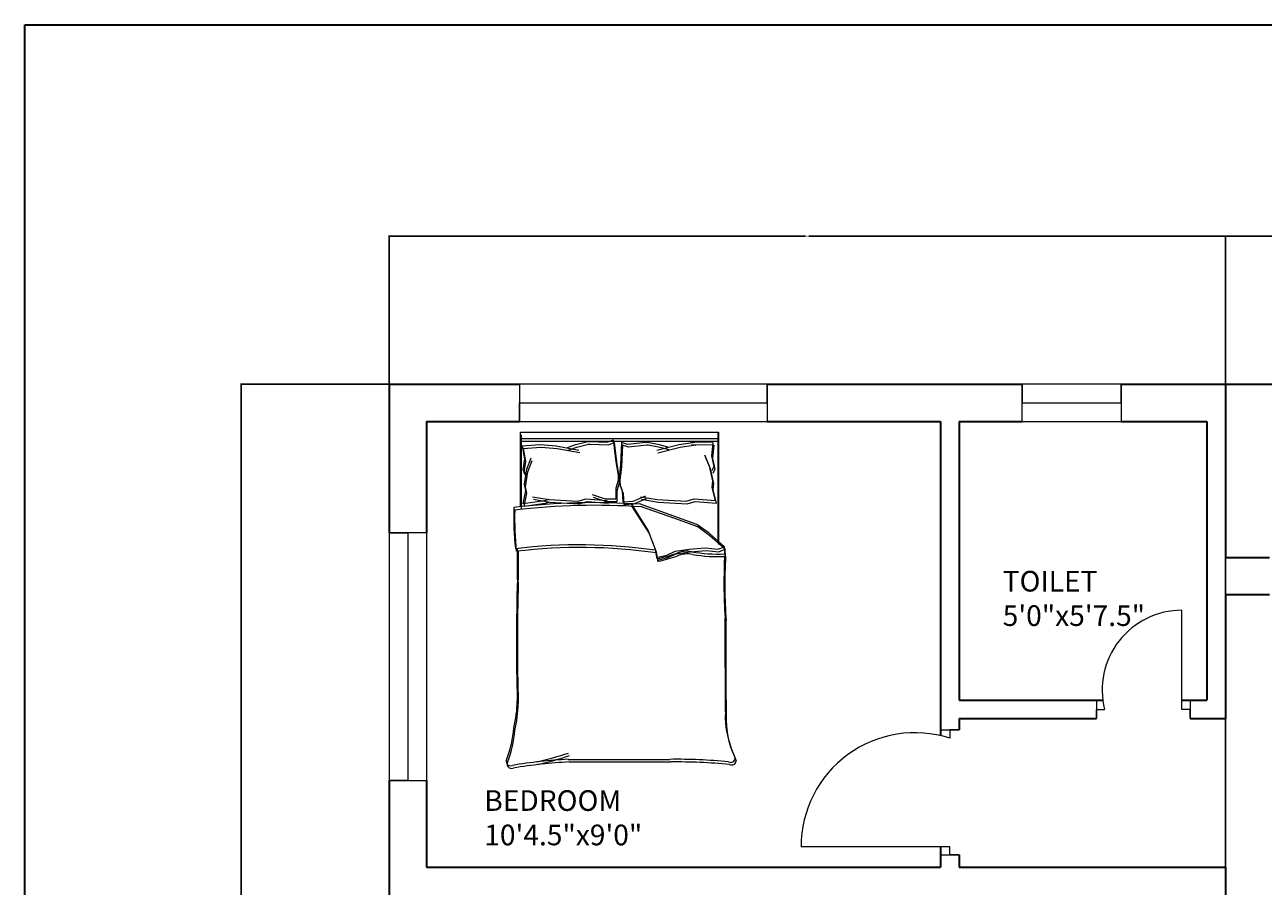
# Model space of a CAD drawing. Units: inches. Extents: x 2527 to 3140, y 1564 to 2435.
# Tile 3 of 4: x 2527 to 2827, y 2227 to 2435. Entities that reach past the tile are written whole.
import ezdxf

# ---------------------------------------------------------------- set-up
doc = ezdxf.new("R2010")
doc.units = ezdxf.units.IN
for name, color, linetype, lineweight in [('A-ANNO-DIMS', 2, 'Continuous', 18), ('A-ANNO-TTLB', 7, 'Continuous', 35), ('A-AREA-IDEN', 7, 'Continuous', 18), ('A-DOOR', 191, 'Continuous', 18), ('A-FURN', 8, 'Continuous', 13), ('A-GLAZ', 131, 'Continuous', 18), ('A-WALL', 7, 'Continuous', 35)]:
    doc.layers.add(name, color=color, linetype=linetype, lineweight=lineweight)
doc.styles.get("Standard").update_dxf_attribs({"font": 'arial.ttf'})
doc.dimstyles.get("Standard").update_dxf_attribs({"dimtxt": 0.18, "dimasz": 0.18, "dimexe": 0.18, "dimexo": 0.0625, "dimgap": 0.09, "dimtad": 0, "dimtih": 1, "dimtoh": 1, "dimdec": 4, "dimzin": 0, "dimdsep": 46, "dimtxsty": 'Standard', "dimcen": 0.09, "dimadec": 0, "dimazin": 0, "dimtfac": 1, "dimtdec": 4, "dimtofl": 0, "dimtmove": 0, "dimatfit": 3, "dimfxl": 1, "dimtolj": 1, "dimtzin": 0, "dimarcsym": 0})

# ---------------------------------------------------------------- blocks, each defined once
blk = doc.blocks.new('BED-DOUBLE')
for p, q in [((3.48, 63.33), (3.48, 81.44)), ((3.48, 63.33), (3.48, 81.44)), ((3.48, 81.44), (51.49, 81.44)), ((51.27, 81.44), (51.27, 54.83)), ((51.27, 81.44), (51.27, 54.83)), ((51.49, 81.44), (51.49, 80.8)), ((3.48, 79.91), (51.27, 79.91)), ((3.48, 79.91), (51.27, 79.91)), ((3.7, 62.69), (3.7, 80.8)), ((3.7, 62.69), (3.7, 80.8)), ((3.7, 79.27), (51.49, 79.27)), ((3.7, 79.27), (51.49, 79.27)), ((3.89, 78.13), (4.47, 74.95)), ((3.9, 78.1), (8.18, 78.43)), ((3.9, 78.1), (8.18, 78.43)), ((3.9, 78.13), (4.47, 74.95)), ((8.18, 78.43), (8.29, 78.42)), ((8.18, 78.43), (8.29, 78.42)), ((8.29, 78.42), (12.11, 78.13)), ((8.29, 78.42), (12.11, 78.13)), ((12.11, 78.13), (17.6, 77.11)), ((12.11, 78.13), (17.6, 77.11)), ((14.86, 77.69), (16.88, 78.42)), ((14.86, 77.69), (16.88, 78.42)), ((16.88, 78.42), (19.77, 79.14)), ((16.88, 78.42), (19.77, 79.14)), ((17.11, 77.78), (20, 78.5)), ((17.11, 77.78), (20, 78.5)), ((19.77, 79.14), (20.09, 79.14)), ((19.77, 79.14), (20.09, 79.14)), ((20, 78.5), (20.32, 78.5)), ((20, 78.5), (20.32, 78.5)), ((20.09, 79.14), (24.54, 78.99)), ((20.09, 79.14), (24.54, 78.99)), ((20.32, 78.5), (24.77, 78.35)), ((20.32, 78.5), (24.77, 78.35)), ((24.54, 78.99), (25.98, 79.57)), ((24.54, 78.99), (25.98, 79.57)), ((24.77, 78.35), (26.21, 78.93)), ((24.77, 78.35), (26.21, 78.93)), ((25.98, 79.57), (26.56, 74.22)), ((25.98, 79.57), (26.56, 74.22)), ((26.21, 78.93), (26.79, 73.58)), ((26.21, 78.93), (26.79, 73.58)), ((27.98, 78.95), (27.73, 73.58)), ((27.98, 78.95), (27.73, 73.58)), ((28.21, 78.31), (27.96, 72.94)), ((28.21, 78.31), (27.96, 72.94)), ((29.46, 78.46), (27.98, 78.95)), ((29.46, 78.46), (27.98, 78.95)), ((29.68, 77.82), (28.21, 78.31)), ((29.68, 77.82), (28.21, 78.31)), ((33.88, 78.89), (29.46, 78.46)), ((33.88, 78.89), (29.46, 78.46)), ((34.11, 78.25), (29.68, 77.82)), ((34.11, 78.25), (29.68, 77.82)), ((34.21, 78.91), (33.88, 78.89)), ((34.2, 78.91), (33.88, 78.89)), ((34.43, 78.27), (34.11, 78.25)), ((34.43, 78.27), (34.11, 78.25)), ((37.14, 78.36), (34.2, 78.91)), ((37.14, 78.36), (34.21, 78.91)), ((37.36, 77.73), (34.43, 78.27)), ((37.36, 77.73), (34.43, 78.27)), ((41.91, 78.37), (36.5, 77.02)), ((41.91, 78.37), (36.5, 77.02)), ((39.2, 77.77), (37.14, 78.36)), ((39.2, 77.77), (37.14, 78.36)), ((45.71, 78.9), (41.91, 78.37)), ((45.71, 78.9), (41.91, 78.37)), ((45.94, 78.26), (42.14, 77.73)), ((45.94, 78.26), (42.14, 77.73)), ((50.11, 78.89), (44.71, 78.98)), ((44.71, 78.98), (45.71, 78.9)), ((50.11, 78.89), (44.71, 78.98)), ((44.71, 78.98), (45.71, 78.9)), ((50.34, 78.25), (44.94, 78.34)), ((44.94, 78.34), (45.94, 78.26)), ((50.34, 78.25), (44.94, 78.34)), ((44.94, 78.34), (45.94, 78.26)), ((50.11, 78.89), (49.73, 75.68)), ((50.11, 78.89), (49.73, 75.68)), ((50.34, 78.25), (49.96, 75.04)), ((50.34, 78.25), (49.96, 75.04)), ((51.49, 80.8), (51.49, 54.19)), ((51.49, 80.8), (51.49, 54.19)), ((4.12, 77.49), (4.7, 74.31)), ((4.12, 77.49), (4.7, 74.31)), ((4.13, 77.47), (8.41, 77.79)), ((4.13, 77.47), (8.41, 77.79)), ((5.05, 72.49), (6.06, 75.24)), ((5.05, 72.49), (6.06, 75.24)), ((8.41, 77.79), (8.51, 77.78)), ((8.41, 77.79), (8.51, 77.78)), ((8.51, 77.78), (12.34, 77.49)), ((8.51, 77.78), (12.34, 77.49)), ((12.34, 77.49), (17.83, 76.48)), ((12.34, 77.49), (17.83, 76.48)), ((15.08, 77.05), (17.11, 77.78)), ((15.08, 77.05), (17.11, 77.78)), ((42.14, 77.73), (36.72, 76.38)), ((42.14, 77.73), (36.72, 76.38)), ((39.43, 77.13), (37.36, 77.73)), ((39.43, 77.13), (37.36, 77.73)), ((49.31, 73.19), (48.13, 75.86)), ((49.31, 73.19), (48.13, 75.86)), ((49.54, 72.55), (48.36, 75.23)), ((49.54, 72.55), (48.36, 75.23)), ((49.73, 75.68), (50.33, 73.1)), ((49.73, 75.68), (50.33, 73.1)), ((49.96, 75.04), (50.56, 72.47)), ((49.96, 75.04), (50.56, 72.47)), ((4.47, 74.95), (4.04, 72.34)), ((4.47, 74.95), (4.04, 72.34)), ((4.04, 72.34), (4.62, 71.33)), ((4.04, 72.34), (4.62, 71.33)), ((4.7, 74.31), (4.27, 71.7)), ((4.7, 74.31), (4.27, 71.7)), ((4.47, 68.87), (5.05, 72.49)), ((4.47, 68.87), (5.05, 72.49)), ((5.28, 71.85), (6.29, 74.6)), ((5.28, 71.85), (6.29, 74.6)), ((26.56, 74.22), (27.14, 71.04)), ((26.56, 74.22), (27.14, 71.04)), ((26.79, 73.58), (27.37, 70.4)), ((26.79, 73.58), (27.37, 70.4)), ((27.73, 73.58), (27.36, 70.36)), ((27.73, 73.58), (27.36, 70.36)), ((27.96, 72.94), (27.58, 69.73)), ((27.96, 72.94), (27.58, 69.73)), ((50.11, 69.61), (49.31, 73.19)), ((50.11, 69.61), (49.31, 73.19)), ((50.34, 68.97), (49.54, 72.55)), ((50.34, 68.97), (49.54, 72.55)), ((50.33, 73.1), (49.81, 72.06)), ((50.33, 73.1), (49.82, 72.06)), ((50.56, 72.47), (50.04, 71.42)), ((50.56, 72.47), (50.04, 71.42)), ((4.27, 71.7), (4.85, 70.69)), ((4.27, 71.7), (4.85, 70.69)), ((4.7, 68.23), (5.28, 71.85)), ((4.7, 68.23), (5.28, 71.85)), ((27.14, 69.74), (26.56, 67.86)), ((27.14, 69.74), (26.56, 67.86)), ((27.37, 69.1), (26.79, 67.22)), ((27.37, 69.1), (26.79, 67.22)), ((27.14, 71.04), (27.14, 69.74)), ((27.14, 71.04), (27.14, 69.74)), ((27.36, 70.36), (27.44, 69.07)), ((27.36, 70.36), (27.44, 69.07)), ((27.37, 70.4), (27.37, 69.1)), ((27.37, 70.4), (27.37, 69.1)), ((27.44, 69.07), (28.13, 67.23)), ((27.44, 69.07), (28.13, 67.23)), ((27.58, 69.73), (27.66, 68.43)), ((27.58, 69.73), (27.66, 68.43)), ((49.92, 68.01), (50.11, 69.61)), ((49.92, 68.01), (50.11, 69.61)), ((4.18, 64.1), (4.76, 67.28)), ((4.18, 64.1), (4.76, 67.28)), ((4.41, 63.46), (4.99, 66.64)), ((4.41, 63.46), (4.99, 66.64)), ((4.76, 67.28), (4.47, 68.87)), ((4.76, 67.28), (4.47, 68.87)), ((4.99, 66.64), (4.7, 68.23)), ((4.99, 66.64), (4.7, 68.23)), ((24.1, 65.18), (20.96, 66.27)), ((24.1, 65.18), (20.96, 66.27)), ((26.56, 67.86), (26.56, 65.18)), ((26.56, 67.86), (26.56, 65.18)), ((26.79, 67.22), (26.79, 64.54)), ((26.79, 67.22), (26.79, 64.54)), ((27.66, 68.43), (28.36, 66.59)), ((27.66, 68.43), (28.36, 66.59)), ((28.13, 67.23), (28.3, 64.55)), ((28.13, 67.23), (28.3, 64.55)), ((28.36, 66.59), (28.53, 63.91)), ((28.36, 66.59), (28.53, 63.91)), ((50.7, 64.87), (49.92, 68.01)), ((50.7, 64.87), (49.92, 68.01)), ((50.15, 67.37), (50.34, 68.97)), ((50.15, 67.37), (50.34, 68.97)), ((50.93, 64.23), (50.15, 67.37)), ((50.93, 64.23), (50.15, 67.37)), ((9.28, 64.82), (4.18, 64.1)), ((9.28, 64.82), (4.18, 64.1)), ((9.51, 64.19), (4.41, 63.46)), ((9.51, 64.19), (4.41, 63.46)), ((6.38, 65.81), (10.41, 65.15)), ((6.38, 65.81), (10.41, 65.15)), ((6.61, 65.17), (10.64, 64.51)), ((6.61, 65.17), (10.64, 64.51)), ((10.41, 65.15), (9.28, 64.82)), ((10.41, 65.15), (9.28, 64.82)), ((10.64, 64.51), (9.51, 64.19)), ((10.64, 64.51), (9.51, 64.19)), ((10.41, 65.15), (17.42, 64.72)), ((10.41, 65.15), (17.42, 64.72)), ((10.64, 64.51), (17.65, 64.08)), ((10.64, 64.51), (17.65, 64.08)), ((17.42, 64.72), (19.38, 65.27)), ((17.42, 64.72), (19.38, 65.27)), ((17.65, 64.08), (19.61, 64.63)), ((17.65, 64.08), (19.61, 64.63)), ((19.38, 65.27), (24.52, 64.87)), ((19.38, 65.27), (24.52, 64.87)), ((19.61, 64.63), (24.74, 64.23)), ((19.61, 64.63), (24.74, 64.23)), ((24.33, 64.54), (21.19, 65.63)), ((24.33, 64.54), (21.19, 65.63)), ((26.56, 65.18), (24.1, 65.18)), ((26.56, 65.18), (24.1, 65.18)), ((26.79, 64.54), (24.33, 64.54)), ((26.79, 64.54), (24.33, 64.54)), ((28.3, 64.55), (30.75, 64.7)), ((28.3, 64.55), (30.75, 64.7)), ((28.53, 63.91), (30.98, 64.06)), ((28.53, 63.91), (30.98, 64.06)), ((30.26, 64.06), (34.45, 57.57)), ((30.26, 64.06), (34.45, 57.57)), ((30.49, 63.42), (34.68, 56.93)), ((30.49, 63.42), (34.68, 56.93)), ((30.75, 64.7), (33.82, 65.99)), ((30.75, 64.7), (33.82, 65.99)), ((30.98, 64.06), (34.05, 65.35)), ((30.98, 64.06), (34.05, 65.35)), ((40.64, 61.13), (32.31, 64.06)), ((40.64, 61.13), (32.31, 64.06)), ((40.87, 60.49), (32.53, 63.42)), ((40.87, 60.49), (32.54, 63.42)), ((32.56, 65.81), (36.6, 65.15)), ((32.56, 65.81), (36.6, 65.15)), ((32.79, 65.17), (36.83, 64.51)), ((32.79, 65.17), (36.82, 64.51)), ((36.6, 65.15), (43.61, 64.72)), ((36.6, 65.15), (43.61, 64.72)), ((36.82, 64.51), (43.83, 64.08)), ((36.83, 64.51), (43.84, 64.08)), ((43.61, 64.72), (45.57, 65.27)), ((43.61, 64.72), (45.57, 65.27)), ((43.83, 64.08), (45.8, 64.63)), ((43.84, 64.08), (45.8, 64.63)), ((45.57, 65.27), (50.7, 64.87)), ((45.57, 65.27), (50.7, 64.87)), ((45.8, 64.63), (50.93, 64.23)), ((45.8, 64.63), (50.93, 64.23)), ((46.22, 59.11), (40.64, 61.13)), ((46.22, 59.11), (40.64, 61.13)), ((46.45, 58.47), (40.87, 60.49)), ((46.45, 58.47), (40.87, 60.49)), ((34.45, 57.57), (36.15, 53.08)), ((34.45, 57.57), (36.15, 53.08)), ((49.16, 56.95), (46.22, 59.11)), ((49.16, 56.95), (46.22, 59.11)), ((49.39, 56.31), (46.45, 58.47)), ((49.39, 56.31), (46.45, 58.47)), ((34.68, 56.93), (36.38, 52.44)), ((34.68, 56.93), (36.38, 52.44)), ((52.87, 53.7), (49.16, 56.95)), ((52.87, 53.7), (49.16, 56.95)), ((53.1, 53.06), (49.39, 56.31)), ((53.1, 53.06), (49.39, 56.31)), ((36.15, 53.08), (36.46, 51.07)), ((36.15, 53.08), (36.46, 51.07)), ((36.38, 52.44), (36.69, 50.43)), ((36.38, 52.44), (36.69, 50.43)), ((36.46, 51.07), (38.94, 51.68)), ((36.46, 51.07), (38.94, 51.68)), ((36.69, 50.43), (39.17, 51.05)), ((36.69, 50.43), (39.17, 51.05)), ((38.94, 51.68), (40.95, 52.61)), ((38.94, 51.68), (40.95, 52.61)), ((39.17, 51.05), (41.18, 51.97)), ((39.17, 51.05), (41.18, 51.97)), ((40.95, 52.61), (44.36, 53.08)), ((40.95, 52.61), (44.36, 53.08)), ((41.18, 51.97), (44.59, 52.44)), ((41.18, 51.97), (44.59, 52.44)), ((44.36, 53.08), (48.23, 53.39)), ((44.36, 53.08), (48.23, 53.39)), ((44.59, 52.44), (48.46, 52.75)), ((44.59, 52.44), (48.46, 52.75)), ((48.23, 53.39), (51.33, 53.08)), ((48.23, 53.39), (51.33, 53.08)), ((48.46, 52.75), (51.56, 52.44)), ((48.46, 52.75), (51.56, 52.44)), ((51.33, 53.08), (52.87, 53.7)), ((51.33, 53.08), (52.87, 53.7)), ((51.56, 52.44), (53.1, 53.06)), ((51.56, 52.44), (53.1, 53.06)), ((52.95, 51.95), (52.87, 53.7, 3.87)), ((52.95, 51.95), (52.87, 53.7, 3.87)), ((53.18, 51.31), (53.1, 53.06, 3.87)), ((53.18, 51.31), (53.1, 53.06, 3.87)), ((15.06, 2.2), (39.68, 2.2)), ((15.06, 2.2), (39.68, 2.2)), ((15.29, 1.56), (39.91, 1.56)), ((15.29, 1.56), (39.91, 1.56))]:
    blk.add_line(p, q)
for centre, radius, start, end in [((85.16, 61.35), 83.31, 178.7218, 185.604), ((85.16, 61.35), 83.31, 178.7218, 185.604), ((21.36, -100.61), 164.97, 86.0865, 96.7821), ((21.36, -100.61), 164.97, 86.0865, 96.7821), ((21.59, -101.25), 164.97, 86.0865, 96.7821), ((21.59, -101.25), 164.97, 86.0865, 96.7821), ((85.39, 60.71), 83.31, 178.7218, 185.604), ((85.39, 60.71), 83.31, 178.7218, 185.604), ((17.76, -74.87), 129.02, 81.7845, 96.9006), ((17.76, -74.87), 129.02, 81.7845, 96.9006), ((17.98, -75.51), 129.02, 81.7845, 96.9006), ((17.98, -75.51), 129.02, 81.7845, 96.9006), ((-167.31, 50.27), 170.11, 358.4762, 1.0082), ((-167.31, 50.27), 170.11, 358.4762, 1.0082), ((-167.08, 49.63), 170.11, 358.4762, 1.0082), ((-167.08, 49.63), 170.11, 358.4762, 1.0082), ((36.64, 51), 0.185, 160.2464, 271.1377), ((36.64, 51), 0.185, 160.2464, 271.1377), ((31.15, 79.96), 29.65, 280.6617, 289.8806), ((31.15, 79.96), 29.65, 280.6617, 289.8806), ((31.38, 79.32), 29.65, 280.6617, 289.8806), ((31.38, 79.32), 29.65, 280.6617, 289.8806), ((43.74, 46.38), 6.22, 78.6608, 113.7384), ((43.74, 46.38), 6.22, 78.6608, 113.7384), ((43.97, 45.74), 6.22, 78.6608, 113.7384), ((43.97, 45.74), 6.22, 78.6608, 113.7384), ((51.33, 88.1), 36.18, 259.8763, 272.5657), ((51.33, 88.1), 36.18, 259.8763, 272.5657), ((51.56, 87.46), 36.18, 259.8763, 272.5657), ((51.56, 87.46), 36.18, 259.8763, 272.5657), ((182.27, 45.13), 129.5, 176.9791, 183.8365), ((182.27, 45.13), 129.5, 176.9791, 183.8365), ((182.49, 44.49), 129.5, 176.9791, 183.8365), ((182.49, 44.49), 129.5, 176.9791, 183.8365), ((36.87, 50.36), 0.185, 160.2464, 271.1377), ((36.86, 50.36), 0.185, 160.2464, 271.1377), ((484.82, 30.83), 482.31, 178.2277, 181.7185), ((484.82, 30.83), 482.31, 178.2277, 181.7185), ((485.05, 30.19), 482.31, 178.2277, 181.7185), ((485.05, 30.19), 482.31, 178.2277, 181.7185), ((-4508.74, 13.62), 4561.86, 0.00217, 0.28689), ((-4508.74, 13.62), 4561.86, 0.00217, 0.28689), ((-4508.51, 12.98), 4561.86, 0.00217, 0.28689), ((-4508.51, 12.98), 4561.86, 0.00217, 0.28689), ((-26.9, 16.93), 29.63, 346.0648, 358.9113), ((-26.9, 16.93), 29.63, 346.0648, 358.9113), ((-26.67, 16.29), 29.63, 346.0648, 358.9113), ((-26.67, 16.29), 29.63, 346.0648, 358.9113), ((76.16, 12.78), 23.07, 177.4714, 206.4681), ((76.16, 12.78), 23.07, 177.4714, 206.4681), ((76.39, 12.14), 23.07, 177.4714, 206.4681), ((76.39, 12.14), 23.07, 177.4714, 206.4681), ((-21.66, 11.17), 23.56, 337.9751, 356.652), ((-21.66, 11.17), 23.56, 337.9751, 356.652), ((-21.43, 10.53), 23.56, 337.9751, 356.652), ((-21.43, 10.53), 23.56, 337.9751, 356.652), ((-17.22, 105.15), 106.46, 283.3832, 287.7053), ((-17.22, 105.15), 106.46, 283.3832, 287.7053), ((-16.99, 104.52), 106.46, 283.3832, 287.7053), ((-16.99, 104.52), 106.46, 283.3832, 287.7053), ((1.09, 1.73), 1.09, 146.1736, 293.4781), ((1.09, 1.73), 1.09, 146.1736, 293.4781), ((1.32, 1.09), 1.09, 146.1736, 293.4781), ((1.32, 1.09), 1.09, 146.1736, 293.4781), ((21.43, -119.39), 121.76, 92.9958, 99.4091), ((21.43, -119.39), 121.76, 92.9958, 99.4091), ((21.66, -120.03), 121.76, 92.9958, 99.4091), ((21.66, -120.03), 121.76, 92.9958, 99.4091), ((41.15, -130.83), 133.04, 84.4998, 90.6351), ((41.15, -130.83), 133.04, 84.4998, 90.6351), ((41.38, -131.47), 133.04, 84.4998, 90.6351), ((41.38, -131.47), 133.04, 84.4998, 90.6351), ((54.41, 2.57), 1.1, 242.6588, 356.02), ((54.41, 2.57), 1.1, 242.6588, 356.02), ((54.64, 1.93), 1.1, 242.6588, 356.02), ((54.64, 1.93), 1.1, 242.6588, 356.02)]:
    blk.add_arc(centre, radius, start, end)
blk = doc.blocks.new('WIN-60')
for p, q in [((0, 9), (0, 0)), ((60, 9), (0, 9)), ((60, 4.5), (60, 9)), ((60, 9), (60, 0)), ((0, 0), (0, 4.5)), ((0, 4.5), (60, 4.5)), ((0, 0), (60, 0))]:
    blk.add_line(p, q)
blk = doc.blocks.new('WIN-24-ALT')
for p, q in [((0, 0), (0, 9)), ((0, 9), (0, 4.5)), ((24, 9), (0, 9)), ((24, 4.5), (24, 9)), ((24, 9), (24, 0)), ((0, 4.5), (24, 4.5)), ((0, 0), (24, 0))]:
    blk.add_line(p, q)
blk = doc.blocks.new('*D20')
at = {"layer": 'A-ANNO-DIMS', "color": 0, "lineweight": -2, "transparency": 16777216}
for p, q in [((2615.52, 2348.14), (2579.55, 2348.14)), ((2579.73, 2347.96), (2579.73, 2027.32)), ((2579.73, 1706.32), (2579.73, 2026.96)), ((2615.52, 1706.14), (2579.55, 1706.14))]:
    blk.add_line(p, q, dxfattribs=at)
at = {"layer": 'A-ANNO-DIMS', "color": 0, "transparency": 16777216}
for points in [[(2579.7, 2347.96), (2579.76, 2347.96), (2579.73, 2348.14)], [(2579.7, 1706.32), (2579.76, 1706.32), (2579.73, 1706.14)]]:
    blk.add_solid(points, dxfattribs=at)
at = {"layer": 'Defpoints', "color": 0, "transparency": 16777216}
for p in [(2579.73, 2348.14), (2615.58, 2348.14), (2615.58, 1706.14)]:
    blk.add_point(p, dxfattribs=at)
at = {"layer": 'A-ANNO-DIMS', "color": 0, "transparency": 16777216, "insert": (2579.73, 2027.14), "char_height": 0.18, "attachment_point": 5}
blk.add_mtext('\\A1;642', dxfattribs=at)
blk = doc.blocks.new('*D21')
at = {"layer": 'A-ANNO-DIMS', "color": 0, "lineweight": -2, "transparency": 16777216}
for p, q in [((2615.58, 2348.21), (2615.58, 2384.17)), ((2615.76, 2383.99), (2716.43, 2383.99)), ((2817.9, 2383.99), (2717.23, 2383.99)), ((2818.08, 2348.21), (2818.08, 2384.17))]:
    blk.add_line(p, q, dxfattribs=at)
at = {"layer": 'A-ANNO-DIMS', "color": 0, "transparency": 16777216}
for points in [[(2615.76, 2384.02), (2615.76, 2383.96), (2615.58, 2383.99)], [(2817.9, 2384.02), (2817.9, 2383.96), (2818.08, 2383.99)]]:
    blk.add_solid(points, dxfattribs=at)
at = {"layer": 'Defpoints', "color": 0, "transparency": 16777216}
for p in [(2818.08, 2383.99), (2615.58, 2348.14), (2818.08, 2348.14)]:
    blk.add_point(p, dxfattribs=at)
at = {"layer": 'A-ANNO-DIMS', "color": 0, "transparency": 16777216, "insert": (2716.83, 2383.99), "char_height": 0.18, "attachment_point": 5}
blk.add_mtext('\\A1;202.5', dxfattribs=at)
blk = doc.blocks.new('*D26')
at = {"layer": 'A-ANNO-DIMS', "color": 0, "lineweight": -2, "transparency": 16777216}
for p, q in [((2818.08, 1994.21), (2818.08, 2384.17)), ((2818.26, 2383.99), (2857.88, 2383.99)), ((2898.29, 2383.99), (2858.67, 2383.99)), ((2898.47, 1994.21), (2898.47, 2384.17))]:
    blk.add_line(p, q, dxfattribs=at)
at = {"layer": 'A-ANNO-DIMS', "color": 0, "transparency": 16777216}
for points in [[(2818.26, 2384.02), (2818.26, 2383.96), (2818.08, 2383.99)], [(2898.29, 2384.02), (2898.29, 2383.96), (2898.47, 2383.99)]]:
    blk.add_solid(points, dxfattribs=at)
at = {"layer": 'Defpoints', "color": 0, "transparency": 16777216}
for p in [(2898.47, 2383.99), (2818.08, 1994.14), (2898.47, 1994.14)]:
    blk.add_point(p, dxfattribs=at)
at = {"layer": 'A-ANNO-DIMS', "color": 0, "transparency": 16777216, "insert": (2858.27, 2383.99), "char_height": 0.18, "attachment_point": 5}
blk.add_mtext('\\A1;80.39', dxfattribs=at)

msp = doc.modelspace()

# ---------------------------------------------------------------- linework, layer by layer
at = {"layer": 'A-ANNO-TTLB'}
msp.add_lwpolyline([(2527.301, 2435.1781), (3140.3962, 2435.1781), (3140.3962, 1564.3652), (2527.301, 1564.3652)], close=True, dxfattribs=at)
at = {"layer": 'A-DOOR'}
for p, q in [((2807.5453, 2269.3926), (2807.5453, 2293.3926)), ((2786.8472, 2271.6426), (2786.8472, 2267.1426)), ((2809.5453, 2271.6426), (2809.5453, 2267.1426)), ((2786.8472, 2267.1426), (2786.8472, 2269.3926)), ((2786.8472, 2269.3926), (2788.8472, 2269.3926)), ((2809.5453, 2269.3926), (2807.5453, 2269.3926)), ((2809.5453, 2267.1426), (2809.5453, 2269.3926)), ((2749.0792, 2264.4315), (2753.5792, 2264.4315)), ((2753.5792, 2264.4315), (2751.3292, 2264.4315)), ((2751.3292, 2264.4315), (2751.3292, 2262.4315)), ((2751.3292, 2236.1364), (2715.3292, 2236.1364)), ((2751.3292, 2234.1364), (2751.3292, 2236.1364)), ((2749.0792, 2234.1364), (2753.5792, 2234.1364)), ((2753.5792, 2234.1364), (2751.3292, 2234.1364))]:
    msp.add_line(p, q, dxfattribs=at)
for centre, radius, start, end in [((2807.5453, 2274.1089), 19.2837, 90, 194.156677), ((2742.9324, 2236.1364), 27.6032, 72.290231, 180)]:
    msp.add_arc(centre, radius, start, end, dxfattribs=at)
at = {"layer": 'A-GLAZ'}
for p, q in [((2624.5792, 2312.1722), (2615.5792, 2312.1722)), ((2615.5792, 2312.1722), (2620.0792, 2312.1722)), ((2615.5792, 2312.1722), (2615.5792, 2252.1722)), ((2620.0792, 2312.1722), (2620.0792, 2252.1722)), ((2624.5792, 2312.1722), (2624.5792, 2252.1722)), ((2620.0792, 2252.1722), (2615.5792, 2252.1722)), ((2615.5792, 2252.1722), (2624.5792, 2252.1722))]:
    msp.add_line(p, q, dxfattribs=at)
at = {"layer": 'A-WALL'}
for p, q in [((2615.5792, 2348.1426), (2647.1466, 2348.1426)), ((2615.5792, 2348.1426), (2647.1466, 2348.1426)), ((2615.5792, 2348.1426), (2615.5792, 2312.1722)), ((2707.1466, 2348.1426), (2768.854, 2348.1426)), ((2707.1466, 2348.1426), (2768.854, 2348.1426)), ((2792.854, 2348.1426), (2818.0792, 2348.1426)), ((2792.854, 2348.1426), (2818.0792, 2348.1426)), ((2818.0792, 2348.1426), (2818.0792, 2306.1426)), ((2818.0792, 2348.1426), (2926.0792, 2348.1426)), ((2818.0792, 2348.1426), (2818.0792, 2306.1426)), ((2624.5792, 2339.1426), (2647.1466, 2339.1426)), ((2624.5792, 2339.1426), (2624.5792, 2312.1722)), ((2707.1466, 2339.1426), (2749.0792, 2339.1426)), ((2749.0792, 2339.1426), (2749.0792, 2263.0466)), ((2753.5792, 2339.1426), (2753.5792, 2271.6426)), ((2753.5792, 2339.1426), (2768.854, 2339.1426)), ((2792.854, 2339.1426), (2813.5792, 2339.1426)), ((2813.5792, 2339.1426), (2813.5792, 2271.6426)), ((2818.0792, 2306.1426), (2828.8027, 2306.1426)), ((2818.0792, 2297.1426), (2818.0792, 2267.1426)), ((2828.8027, 2297.1426), (2818.0792, 2297.1426)), ((2753.5792, 2271.6426), (2788.42, 2271.6426)), ((2807.5453, 2271.6426), (2813.5792, 2271.6426)), ((2753.5792, 2267.1426), (2786.8472, 2267.1426)), ((2753.5792, 2267.1426), (2753.5792, 2264.4315)), ((2809.5453, 2267.1426), (2818.0792, 2267.1426)), ((2615.5792, 2252.1722), (2615.5792, 2217.785)), ((2624.5792, 2252.1722), (2624.5792, 2231.1426)), ((2749.0792, 2236.1364), (2749.0792, 2231.1426)), ((2753.5792, 2234.1364), (2753.5792, 2231.1426)), ((2624.5792, 2231.1426), (2749.0792, 2231.1426)), ((2753.5792, 2231.1426), (2818.0792, 2231.1426)), ((2818.0792, 2231.1426), (2818.0792, 2075.1426))]:
    msp.add_line(p, q, dxfattribs=at)

# ---------------------------------------------------------------- block references
at = {"layer": 'A-FURN'}
msp.add_blockref('BED-DOUBLE', (2643.87, 2255.088), dxfattribs=at)
at = {"layer": 'A-GLAZ'}
for name, p in [('WIN-60', (2647.147, 2339.143)), ('WIN-24-ALT', (2768.854, 2339.143))]:
    msp.add_blockref(name, p, dxfattribs=at)

# ---------------------------------------------------------------- texts
at = {"layer": 'A-AREA-IDEN', "char_height": 5, "attachment_point": 1}
for s, width, insert in [('TOILET\\P5\'0"x5\'7.5"', 118.765491, (2764.1542, 2302.926)), ('BEDROOM\\P10\'4.5"x9\'0"', 128.382992, (2638.5908, 2249.8049))]:
    msp.add_mtext_dynamic_manual_height_columns(s, width=width, gutter_width=12.5, heights=[0], dxfattribs=dict(at, insert=insert))

# ---------------------------------------------------------------- dimensions: what is measured, and where the dimension line sits
at = {"layer": 'A-ANNO-DIMS'}
for base, p1, p2, override, picture, middle in [((2818.0792, 2383.9926), (2615.5792, 2348.1426), (2818.0792, 2348.1426), {"dimdec": 1, "dimlfac": 1, "dimrnd": 0, "dimzin": 0, "dimdsep": 46, "dimlunit": 2}, '*D21', (2716.8292, 2383.9926)), ((2898.4651, 2383.9926), (2818.0792, 1994.1426), (2898.4651, 1994.1426), {"dimdec": 2, "dimlfac": 1, "dimrnd": 0, "dimzin": 0, "dimdsep": 46, "dimlunit": 2}, '*D26', (2858.2722, 2383.9926))]:
    dim = msp.add_linear_dim(base=base, p1=p1, p2=p2, dimstyle='Standard', override=override, dxfattribs=at)
    dim.commit()
    dim.dimension.update_dxf_attribs({"geometry": picture, "text_midpoint": middle})
dim = msp.add_linear_dim(base=(2579.7292, 2348.1426), p1=(2615.5792, 1706.1426), p2=(2615.5792, 2348.1426), angle=90, dimstyle='Standard', override={"dimdec": 0, "dimlfac": 1, "dimrnd": 0, "dimzin": 0, "dimdsep": 46, "dimlunit": 2}, dxfattribs=at)
dim.commit()
dim.dimension.update_dxf_attribs({"geometry": '*D20', "text_midpoint": (2579.7292, 2027.1426)})

doc.saveas('drawing.dxf')
